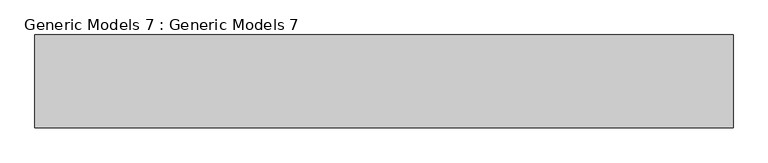
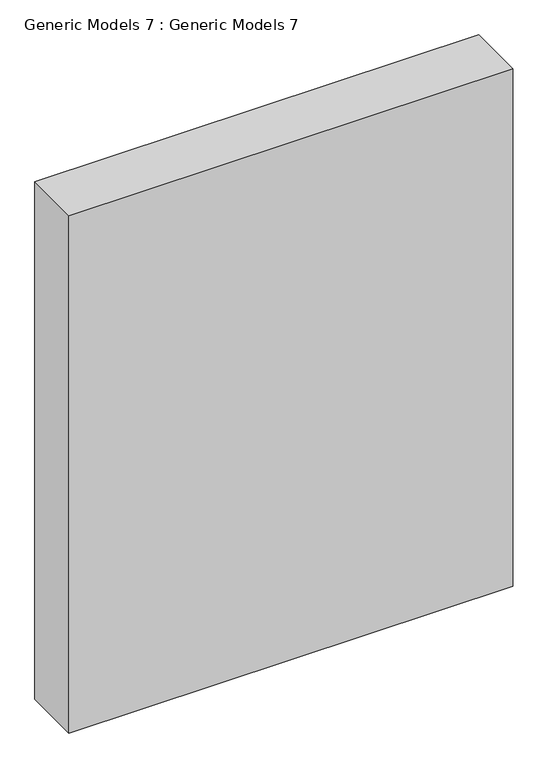
"""IFC4 building model written with IfcOpenShell, lengths in millimetres: proxy geometry, Generic Models 7 : Generic Models 7."""

from ifc_helpers import new_model, si_unit, frame, origin, place, context, project, spatial, polyline, outline, extrude, source, transform, mapped, element, save


def generic_models_7_generic_models_7_2f98df86(model_context):
    return source(origin(), model_context, "Body", "SweptSolid", [
        extrude(outline(polyline([(-6735.102412, -14738.7800298), (-5107.5321088, -14738.7800298), (-5107.5321088, -14954.9057689), (-6735.102412, -14954.9057689), (-6735.102412, -14738.7800298)])), frame((0.0, 0.0, 4089.4), z_axis=(0.0, 0.0, 1.0), x_axis=(1.0, 0.0, 0.0)), (0.0, 0.0, 1.0), 2006.6),
    ])


if __name__ == "__main__":
    model = new_model("IFC4")
    model_context = context("Model", 3, world=origin())
    ifc_project = project(units=[si_unit("LENGTHUNIT", "METRE", prefix="MILLI")], contexts=[model_context])
    site = spatial("IfcSite", under=ifc_project)
    building = spatial("IfcBuilding", under=site)
    placement = place(None, origin())
    generic_models_7_generic_models_7_shape = generic_models_7_generic_models_7_2f98df86(model_context)
    element("IfcBuildingElementProxy", 1, Name="Generic Models 7 : Generic Models 7", ObjectType="Generic Models 7 : Generic Models 7", at=placement, inside=building, context=model_context, shape_type="MappedRepresentation", body=[
        mapped(generic_models_7_generic_models_7_shape, transform((0.0, 0.0, 0.0), x_axis=(1.0, 0.0, 0.0), y_axis=(0.0, 1.0, 0.0), z_axis=(0.0, 0.0, 1.0))),
    ])
    save(model, "model.ifc")
